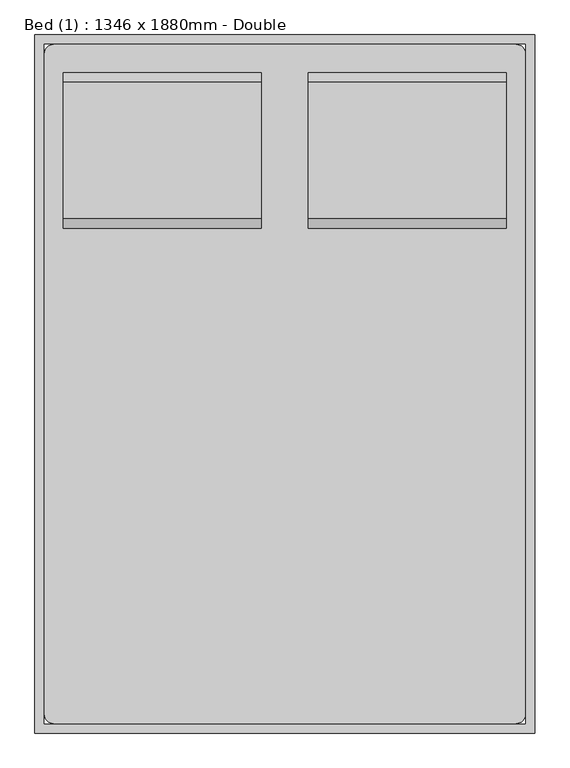
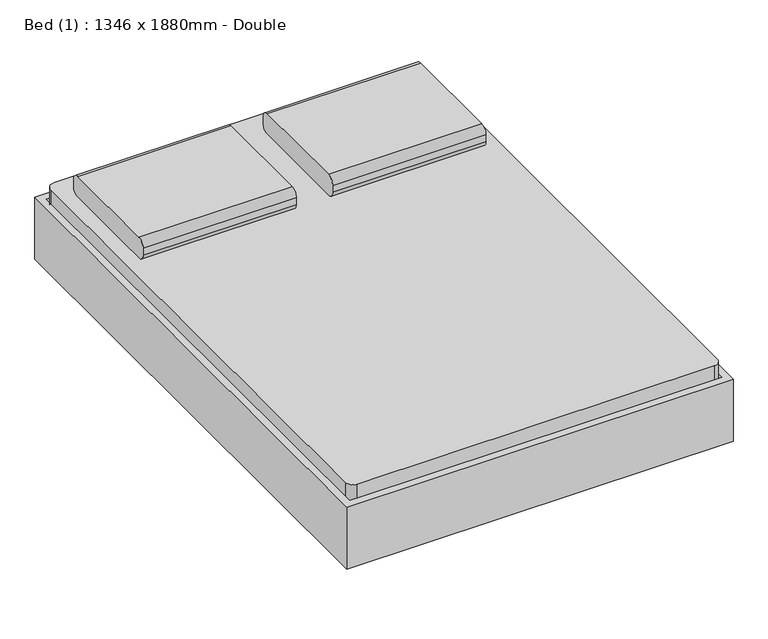
"""IFC4 building model written with IfcOpenShell, lengths in millimetres: furniture geometry, Bed (1) : 1346 x 1880mm - Double."""

from ifc_helpers import new_model, si_unit, point, frame, frame_2d, origin, place, context, project, spatial, polyline, circle_curve, trimmed, segment, composite_curve, outline, extrude, source, transform, mapped, element, save
from ifc_brep_helpers import plane_surface, cylinder_surface, revolved_surface, advanced_brep


def bed_1_1346_x_1880mm_double_99e58f25(model_context):
    return source(origin(), model_context, "Body", "SolidModel", [
        advanced_brep(
        [(-308.447541, -869.6295082, 196.85), (-308.447541, -869.6295082, 177.8), (-308.447541, -945.8295082, 177.8), (-308.447541, -945.8295082, 196.85), (-245.5113525, -869.6295082, 196.85), (-257.647541, -869.6295082, 177.8), (-257.647541, -945.8295082, 177.8), (-245.5113525, -945.8295082, 196.85), (-164.3115092, -869.6295082, 22.716374), (-181.5766725, -869.6295082, 14.6654962), (-181.5766725, -945.8295082, 14.6654962), (-164.3115092, -945.8295082, 22.716374), (-158.5564547, -869.6295082, 0.0), (-158.5564547, -869.6295082, 19.05), (-158.5564547, -945.8295082, 0.0), (-158.5564547, -945.8295082, 19.05), (-79.9439489, -869.6295082, 19.05), (-79.9439489, -869.6295082, 0.0), (-79.9439489, -945.8295082, 0.0), (-79.9439489, -945.8295082, 19.05), (-67.2439489, -869.6295082, 3.4029547), (-76.7689489, -869.6295082, 19.9007387), (-67.2439489, -945.8295082, 3.4029547), (-76.7689489, -945.8295082, 19.9007387), (-12.2513357, -869.6295082, 57.15), (-7.1469036, -869.6295082, 38.1), (-7.1469036, -945.8295082, 38.1), (-12.2513357, -945.8295082, 57.15), (690.5562537, -869.6295082, 57.15), (685.4518216, -869.6295082, 38.1), (685.4518216, -945.8295082, 38.1), (690.5562537, -945.8295082, 57.15), (755.0738669, -869.6295082, 19.9007387), (745.5488669, -869.6295082, 3.4029547), (745.5488669, -945.8295082, 3.4029547), (755.0738669, -945.8295082, 19.9007387), (758.2488669, -869.6295082, 0.0), (758.2488669, -869.6295082, 19.05), (758.2488669, -945.8295082, 0.0), (758.2488669, -945.8295082, 19.05), (836.8613728, -869.6295082, 19.05), (836.8613728, -869.6295082, 0.0), (836.8613728, -945.8295082, 0.0), (836.8613728, -945.8295082, 19.05), (859.8815906, -869.6295082, 14.6654962), (842.6164272, -869.6295082, 22.716374), (859.8815906, -945.8295082, 14.6654962), (842.6164272, -945.8295082, 22.716374), (923.8162705, -869.6295082, 196.85), (935.952459, -869.6295082, 177.8), (935.952459, -945.8295082, 177.8), (923.8162705, -945.8295082, 196.85), (986.752459, -869.6295082, 196.85), (986.752459, -945.8295082, 196.85), (986.752459, -945.8295082, 177.8), (986.752459, -869.6295082, 177.8)],
        [
            (0, 1),
            (1, 2),
            (2, 3),
            (3, 0),
            (0, 4),
            (4, 5),
            (5, 1),
            (5, 6),
            (6, 2),
            (6, 7),
            (7, 3),
            (7, 4),
            (4, 8),
            (8, 9),
            (9, 5),
            (9, 10),
            (10, 6),
            (10, 11),
            (11, 7),
            (11, 8),
            (12, 9, circle_curve(frame((-158.5564547, -869.6295082, 25.4), z_axis=(0.0, 1.0, 0.0), x_axis=(-0.906307787036664, 0.0, -0.4226182617406693)), 25.4)),
            (8, 13, circle_curve(frame((-158.5564547, -869.6295082, 25.4), z_axis=(0.0, -1.0, 0.0), x_axis=(-0.906307787036664, 0.0, -0.4226182617406693)), 6.35)),
            (13, 12),
            (14, 10, circle_curve(frame((-158.5564547, -945.8295082, 25.4), z_axis=(0.0, 1.0, 0.0), x_axis=(-0.906307787036664, 0.0, -0.4226182617406693)), 25.4)),
            (12, 14),
            (15, 11, circle_curve(frame((-158.5564547, -945.8295082, 25.4), z_axis=(0.0, 1.0, 0.0), x_axis=(-0.906307787036664, 0.0, -0.4226182617406693)), 6.35)),
            (14, 15),
            (15, 13),
            (13, 16),
            (16, 17),
            (17, 12),
            (17, 18),
            (18, 14),
            (18, 19),
            (19, 15),
            (19, 16),
            (20, 17, circle_curve(frame((-79.9439489, -869.6295082, 25.4), z_axis=(0.0, 1.0, 0.0), x_axis=(0.0, 0.0, -1.0)), 25.4)),
            (16, 21, circle_curve(frame((-79.9439489, -869.6295082, 25.4), z_axis=(0.0, -1.0, 0.0), x_axis=(0.0, 0.0, -1.0)), 6.35)),
            (21, 20),
            (22, 18, circle_curve(frame((-79.9439489, -945.8295082, 25.4), z_axis=(0.0, 1.0, 0.0), x_axis=(0.0, 0.0, -1.0)), 25.4)),
            (20, 22),
            (23, 19, circle_curve(frame((-79.9439489, -945.8295082, 25.4), z_axis=(0.0, 1.0, 0.0), x_axis=(0.0, 0.0, -1.0)), 6.35)),
            (22, 23),
            (23, 21),
            (21, 24),
            (24, 25),
            (25, 20),
            (25, 26),
            (26, 22),
            (26, 27),
            (27, 23),
            (27, 24),
            (24, 28),
            (28, 29),
            (29, 25),
            (29, 30),
            (30, 26),
            (30, 31),
            (31, 27),
            (31, 28),
            (28, 32),
            (32, 33),
            (33, 29),
            (33, 34),
            (34, 30),
            (34, 35),
            (35, 31),
            (35, 32),
            (36, 33, circle_curve(frame((758.2488669, -869.6295082, 25.4), z_axis=(0.0, 1.0, 0.0), x_axis=(-0.5000000000000533, 0.0, -0.866025403784408)), 25.4)),
            (32, 37, circle_curve(frame((758.2488669, -869.6295082, 25.4), z_axis=(0.0, -1.0, 0.0), x_axis=(-0.5000000000000533, 0.0, -0.866025403784408)), 6.35)),
            (37, 36),
            (38, 34, circle_curve(frame((758.2488669, -945.8295082, 25.4), z_axis=(0.0, 1.0, 0.0), x_axis=(-0.5000000000000533, 0.0, -0.866025403784408)), 25.4)),
            (36, 38),
            (39, 35, circle_curve(frame((758.2488669, -945.8295082, 25.4), z_axis=(0.0, 1.0, 0.0), x_axis=(-0.5000000000000533, 0.0, -0.866025403784408)), 6.35)),
            (38, 39),
            (39, 37),
            (37, 40),
            (40, 41),
            (41, 36),
            (41, 42),
            (42, 38),
            (42, 43),
            (43, 39),
            (43, 40),
            (44, 41, circle_curve(frame((836.8613728, -869.6295082, 25.4), z_axis=(0.0, 1.0, 0.0), x_axis=(0.0, 0.0, -1.0)), 25.4)),
            (40, 45, circle_curve(frame((836.8613728, -869.6295082, 25.4), z_axis=(0.0, -1.0, 0.0), x_axis=(0.0, 0.0, -1.0)), 6.35)),
            (45, 44),
            (46, 42, circle_curve(frame((836.8613728, -945.8295082, 25.4), z_axis=(0.0, 1.0, 0.0), x_axis=(0.0, 0.0, -1.0)), 25.4)),
            (44, 46),
            (47, 43, circle_curve(frame((836.8613728, -945.8295082, 25.4), z_axis=(0.0, 1.0, 0.0), x_axis=(0.0, 0.0, -1.0)), 6.35)),
            (46, 47),
            (47, 45),
            (45, 48),
            (48, 49),
            (49, 44),
            (49, 50),
            (50, 46),
            (50, 51),
            (51, 47),
            (51, 48),
            (52, 53),
            (53, 54),
            (54, 55),
            (55, 52),
            (48, 52),
            (55, 49),
            (54, 50),
            (53, 51),
        ],
        [
            plane_surface(frame((-308.447541, -1174.4295082, -127.5947323), z_axis=(-1.0, 0.0, 0.0), x_axis=(0.0, 1.0, 0.0))),
            plane_surface(frame((-308.447541, -869.6295082, 196.85), z_axis=(0.0, 1.0, 0.0), x_axis=(1.0, 0.0, 0.0))),
            plane_surface(frame((-308.447541, -869.6295082, 177.8), z_axis=(0.0, 0.0, -1.0), x_axis=(1.0, 0.0, 0.0))),
            plane_surface(frame((-308.447541, -945.8295082, 177.8), z_axis=(0.0, -1.0, 0.0), x_axis=(1.0, 0.0, 0.0))),
            plane_surface(frame((-308.447541, -945.8295082, 196.85), z_axis=(0.0, 0.0, 1.0), x_axis=(1.0, 0.0, 0.0))),
            plane_surface(frame((-245.5113525, -869.6295082, 196.85), z_axis=(0.0, 1.0000000000000002, 0.0), x_axis=(0.4226182617406713, 0.0, -0.9063077870366631))),
            plane_surface(frame((-257.647541, -869.6295082, 177.8), z_axis=(-0.9063077870366631, 0.0, -0.4226182617406712), x_axis=(0.4226182617406712, 0.0, -0.9063077870366631))),
            plane_surface(frame((-257.647541, -945.8295082, 177.8), z_axis=(0.0, -1.0000000000000002, 0.0), x_axis=(0.4226182617406716, 0.0, -0.906307787036663))),
            plane_surface(frame((-245.5113525, -945.8295082, 196.85), z_axis=(0.906307787036663, 0.0, 0.4226182617406715), x_axis=(0.4226182617406715, 0.0, -0.906307787036663))),
            plane_surface(frame((-158.5564547, -869.6295082, 25.4), z_axis=(0.0, 1.0, 0.0), x_axis=(-0.906307787036664, 0.0, -0.4226182617406693))),
            cylinder_surface(frame((-158.5564547, -1174.4295082, 25.4), z_axis=(0.0, -1.0, 0.0), x_axis=(-0.906307787036664, 0.0, -0.4226182617406693)), 25.4),
            plane_surface(frame((-158.5564547, -945.8295082, 25.4), z_axis=(0.0, -1.0, 0.0), x_axis=(-0.906307787036664, 0.0, -0.4226182617406693))),
            revolved_surface(polyline([(-164.3115091476828, -945.8295082, 22.71637403794675), (-164.3115091476828, -869.6295082, 22.71637403794675)]), (-158.5564547, -1174.4295082, 25.4), (0.0, -1.0, 0.0)),
            plane_surface(frame((-158.5564547, -869.6295082, 19.05), z_axis=(0.0, 1.0, 0.0), x_axis=(1.0, 0.0, 0.0))),
            plane_surface(frame((-158.5564547, -869.6295082, 0.0), z_axis=(0.0, 0.0, -1.0), x_axis=(1.0, 0.0, 0.0))),
            plane_surface(frame((-158.5564547, -945.8295082, 0.0), z_axis=(0.0, -1.0, 0.0), x_axis=(1.0, 0.0, 0.0))),
            plane_surface(frame((-158.5564547, -945.8295082, 19.05), z_axis=(0.0, 0.0, 1.0), x_axis=(1.0, 0.0, 0.0))),
            plane_surface(frame((-79.9439489, -869.6295082, 25.4), z_axis=(0.0, 1.0, 0.0), x_axis=(0.0, 0.0, -1.0))),
            cylinder_surface(frame((-79.9439489, -1174.4295082, 25.4), z_axis=(0.0, -1.0, 0.0), x_axis=(0.0, 0.0, -1.0)), 25.4),
            plane_surface(frame((-79.9439489, -945.8295082, 25.4), z_axis=(0.0, -1.0, 0.0), x_axis=(0.0, 0.0, -1.0))),
            revolved_surface(polyline([(-79.9439489, -945.8295082, 19.049999999999997), (-79.9439489, -869.6295082, 19.049999999999997)]), (-79.9439489, -1174.4295082, 25.4), (0.0, -1.0, 0.0)),
            plane_surface(frame((-76.7689489, -869.6295082, 19.9007387), z_axis=(0.0, 1.0, 0.0), x_axis=(0.8660254037844781, 0.0, 0.4999999999999317))),
            plane_surface(frame((-67.2439489, -869.6295082, 3.4029547), z_axis=(0.4999999999999313, 0.0, -0.8660254037844783), x_axis=(0.8660254037844783, 0.0, 0.4999999999999313))),
            plane_surface(frame((-67.2439489, -945.8295082, 3.4029547), z_axis=(0.0, -1.0000000000000002, 0.0), x_axis=(0.8660254037844788, 0.0, 0.49999999999993067))),
            plane_surface(frame((-76.7689489, -945.8295082, 19.9007387), z_axis=(-0.49999999999993067, 0.0, 0.8660254037844787), x_axis=(0.8660254037844787, 0.0, 0.49999999999993067))),
            plane_surface(frame((-12.2513357, -869.6295082, 57.15), z_axis=(0.0, 1.0, 0.0), x_axis=(1.0, 0.0, 0.0))),
            plane_surface(frame((-7.1469036, -869.6295082, 38.1), z_axis=(0.0, 0.0, -1.0), x_axis=(1.0, 0.0, 0.0))),
            plane_surface(frame((-7.1469036, -945.8295082, 38.1), z_axis=(0.0, -1.0, 0.0), x_axis=(1.0, 0.0, 0.0))),
            plane_surface(frame((-12.2513357, -945.8295082, 57.15), z_axis=(0.0, 0.0, 1.0), x_axis=(1.0, 0.0, 0.0))),
            plane_surface(frame((690.5562537, -869.6295082, 57.15), z_axis=(0.0, 1.0, 0.0), x_axis=(0.8660254037844102, 0.0, -0.5000000000000493))),
            plane_surface(frame((685.4518216, -869.6295082, 38.1), z_axis=(-0.500000000000049, 0.0, -0.8660254037844105), x_axis=(0.8660254037844105, 0.0, -0.500000000000049))),
            plane_surface(frame((685.4518216, -945.8295082, 38.1), z_axis=(0.0, -1.0, 0.0), x_axis=(0.8660254037844105, 0.0, -0.5000000000000488))),
            plane_surface(frame((690.5562537, -945.8295082, 57.15), z_axis=(0.5000000000000491, 0.0, 0.8660254037844103), x_axis=(0.8660254037844103, 0.0, -0.5000000000000491))),
            plane_surface(frame((758.2488669, -869.6295082, 25.4), z_axis=(0.0, 1.0, 0.0), x_axis=(-0.5000000000000533, 0.0, -0.866025403784408))),
            cylinder_surface(frame((758.2488669, -1174.4295082, 25.4), z_axis=(0.0, -1.0, 0.0), x_axis=(-0.5000000000000533, 0.0, -0.866025403784408)), 25.4),
            plane_surface(frame((758.2488669, -945.8295082, 25.4), z_axis=(0.0, -1.0, 0.0), x_axis=(-0.5000000000000533, 0.0, -0.866025403784408))),
            revolved_surface(polyline([(755.0738668999998, -945.8295082, 19.90073868596901), (755.0738668999998, -869.6295082, 19.90073868596901)]), (758.2488669, -1174.4295082, 25.4), (0.0, -1.0, 0.0)),
            plane_surface(frame((758.2488669, -869.6295082, 19.05), z_axis=(0.0, 1.0, 0.0), x_axis=(1.0, 0.0, 0.0))),
            plane_surface(frame((758.2488669, -869.6295082, 0.0), z_axis=(0.0, 0.0, -1.0), x_axis=(1.0, 0.0, 0.0))),
            plane_surface(frame((758.2488669, -945.8295082, 0.0), z_axis=(0.0, -1.0, 0.0), x_axis=(1.0, 0.0, 0.0))),
            plane_surface(frame((758.2488669, -945.8295082, 19.05), z_axis=(0.0, 0.0, 1.0), x_axis=(1.0, 0.0, 0.0))),
            plane_surface(frame((836.8613728, -869.6295082, 25.4), z_axis=(0.0, 1.0, 0.0), x_axis=(0.0, 0.0, -1.0))),
            cylinder_surface(frame((836.8613728, -1174.4295082, 25.4), z_axis=(0.0, -1.0, 0.0), x_axis=(0.0, 0.0, -1.0)), 25.4),
            plane_surface(frame((836.8613728, -945.8295082, 25.4), z_axis=(0.0, -1.0, 0.0), x_axis=(0.0, 0.0, -1.0))),
            revolved_surface(polyline([(836.8613728, -945.8295082, 19.049999999999997), (836.8613728, -869.6295082, 19.049999999999997)]), (836.8613728, -1174.4295082, 25.4), (0.0, -1.0, 0.0)),
            plane_surface(frame((842.6164272, -869.6295082, 22.716374), z_axis=(0.0, 1.0000000000000002, 0.0), x_axis=(0.42261826174054035, 0.0, 0.9063077870367242))),
            plane_surface(frame((859.8815906, -869.6295082, 14.6654962), z_axis=(0.9063077870367245, 0.0, -0.42261826174053974), x_axis=(0.42261826174053974, 0.0, 0.9063077870367245))),
            plane_surface(frame((859.8815906, -945.8295082, 14.6654962), z_axis=(0.0, -1.0, 0.0), x_axis=(0.42261826174053996, 0.0, 0.9063077870367243))),
            plane_surface(frame((842.6164272, -945.8295082, 22.716374), z_axis=(-0.9063077870367245, 0.0, 0.4226182617405396), x_axis=(0.4226182617405396, 0.0, 0.9063077870367245))),
            plane_surface(frame((986.752459, -1174.4295082, -127.5947323), z_axis=(1.0, 0.0, 0.0), x_axis=(0.0, 1.0, 0.0))),
            plane_surface(frame((923.8162705, -869.6295082, 196.85), z_axis=(0.0, 1.0, 0.0), x_axis=(1.0, 0.0, 0.0))),
            plane_surface(frame((935.952459, -869.6295082, 177.8), z_axis=(0.0, 0.0, -1.0), x_axis=(1.0, 0.0, 0.0))),
            plane_surface(frame((935.952459, -945.8295082, 177.8), z_axis=(0.0, -1.0, 0.0), x_axis=(1.0, 0.0, 0.0))),
            plane_surface(frame((923.8162705, -945.8295082, 196.85), z_axis=(0.0, 0.0, 1.0), x_axis=(1.0, 0.0, 0.0))),
        ],
        [
            (0, [[1, 2, 3, 4]]),
            (1, [[-1, 5, 6, 7]]),
            (2, [[-2, -7, 8, 9]]),
            (3, [[-3, -9, 10, 11]]),
            (4, [[-4, -11, 12, -5]]),
            (5, [[-6, 13, 14, 15]]),
            (6, [[-8, -15, 16, 17]]),
            (7, [[-10, -17, 18, 19]]),
            (8, [[-12, -19, 20, -13]]),
            (9, [[21, -14, 22, 23]]),
            (10, [[24, -16, -21, 25]]),
            (11, [[26, -18, -24, 27]]),
            (12, [[-22, -20, -26, 28]]),
            (13, [[-23, 29, 30, 31]]),
            (14, [[-25, -31, 32, 33]]),
            (15, [[-27, -33, 34, 35]]),
            (16, [[-28, -35, 36, -29]]),
            (17, [[37, -30, 38, 39]]),
            (18, [[40, -32, -37, 41]]),
            (19, [[42, -34, -40, 43]]),
            (20, [[-38, -36, -42, 44]]),
            (21, [[-39, 45, 46, 47]]),
            (22, [[-41, -47, 48, 49]]),
            (23, [[-43, -49, 50, 51]]),
            (24, [[-44, -51, 52, -45]]),
            (25, [[-46, 53, 54, 55]]),
            (26, [[-48, -55, 56, 57]]),
            (27, [[-50, -57, 58, 59]]),
            (28, [[-52, -59, 60, -53]]),
            (29, [[-54, 61, 62, 63]]),
            (30, [[-56, -63, 64, 65]]),
            (31, [[-58, -65, 66, 67]]),
            (32, [[-60, -67, 68, -61]]),
            (33, [[69, -62, 70, 71]]),
            (34, [[72, -64, -69, 73]]),
            (35, [[74, -66, -72, 75]]),
            (36, [[-70, -68, -74, 76]]),
            (37, [[-71, 77, 78, 79]]),
            (38, [[-73, -79, 80, 81]]),
            (39, [[-75, -81, 82, 83]]),
            (40, [[-76, -83, 84, -77]]),
            (41, [[85, -78, 86, 87]]),
            (42, [[88, -80, -85, 89]]),
            (43, [[90, -82, -88, 91]]),
            (44, [[-86, -84, -90, 92]]),
            (45, [[-87, 93, 94, 95]]),
            (46, [[-89, -95, 96, 97]]),
            (47, [[-91, -97, 98, 99]]),
            (48, [[-92, -99, 100, -93]]),
            (49, [[101, 102, 103, 104]]),
            (50, [[-94, 105, -104, 106]]),
            (51, [[-96, -106, -103, 107]]),
            (52, [[-98, -107, -102, 108]]),
            (53, [[-100, -108, -101, -105]]),
        ],
    ),
        extrude(outline(composite_curve([segment(polyline([(-283.047541, 680.1704918), (961.352459, 680.1704918)]), True, "CONTINUOUS"), segment(trimmed(circle_curve(frame_2d((961.352459, 654.7704918)), 25.4), [point((961.352459, 680.1704918))], [point((986.752459, 654.7704918))], False, "CARTESIAN"), True, "CONTINUOUS"), segment(polyline([(986.752459, 654.7704918), (986.752459, -1123.6295082)]), True, "CONTINUOUS"), segment(trimmed(circle_curve(frame_2d((961.352459, -1123.6295082)), 25.4), [point((986.752459, -1123.6295082))], [point((961.352459, -1149.0295082))], False, "CARTESIAN"), True, "CONTINUOUS"), segment(polyline([(961.352459, -1149.0295082), (-283.047541, -1149.0295082)]), True, "CONTINUOUS"), segment(trimmed(circle_curve(frame_2d((-283.047541, -1123.6295082)), 25.4), [point((-283.047541, -1149.0295082))], [point((-308.447541, -1123.6295082))], False, "CARTESIAN"), True, "CONTINUOUS"), segment(polyline([(-308.447541, -1123.6295082), (-308.447541, 654.7704918)]), True, "CONTINUOUS"), segment(trimmed(circle_curve(frame_2d((-283.047541, 654.7704918)), 25.4), [point((-308.447541, 654.7704918))], [point((-283.047541, 680.1704918))], False, "CARTESIAN"), True, "CONTINUOUS")], self_intersect=False)), frame((0.0, 0.0, 203.2), z_axis=(0.0, 0.0, 1.0), x_axis=(1.0, 0.0, 0.0)), (0.0, 0.0, 1.0), 203.2),
        advanced_brep(
        [(-308.1231784, 451.5704918, 177.8), (-308.1231784, 375.3704918, 177.8), (-308.1231784, 375.3704918, 196.85), (-308.1231784, 451.5704918, 196.85), (-257.3231784, 451.5704918, 177.8), (-257.3231784, 375.3704918, 177.8), (-245.1869899, 375.3704918, 196.85), (-245.1869899, 451.5704918, 196.85), (-181.2523099, 451.5704918, 14.6654962), (-181.2523099, 375.3704918, 14.6654962), (-163.9871466, 375.3704918, 22.716374), (-163.9871466, 451.5704918, 22.716374), (-158.2320921, 375.3704918, 0.0), (-158.2320921, 451.5704918, 0.0), (-158.2320921, 375.3704918, 19.05), (-158.2320921, 451.5704918, 19.05), (-79.6195862, 451.5704918, 0.0), (-79.6195862, 375.3704918, 0.0), (-79.6195862, 375.3704918, 19.05), (-79.6195862, 451.5704918, 19.05), (-66.9195862, 375.3704918, 3.4029547), (-66.9195862, 451.5704918, 3.4029547), (-76.4445862, 375.3704918, 19.9007387), (-76.4445862, 451.5704918, 19.9007387), (-6.822541, 451.5704918, 38.1), (-6.822541, 375.3704918, 38.1), (-11.9269731, 375.3704918, 57.15), (-11.9269731, 451.5704918, 57.15), (685.4518216, 451.5704918, 38.1), (685.4518216, 375.3704918, 38.1), (690.5562537, 375.3704918, 57.15), (690.5562537, 451.5704918, 57.15), (745.5488669, 451.5704918, 3.4029547), (745.5488669, 375.3704918, 3.4029547), (755.0738669, 375.3704918, 19.9007387), (755.0738669, 451.5704918, 19.9007387), (758.2488669, 375.3704918, 0.0), (758.2488669, 451.5704918, 0.0), (758.2488669, 375.3704918, 19.05), (758.2488669, 451.5704918, 19.05), (836.8613728, 451.5704918, 0.0), (836.8613728, 375.3704918, 0.0), (836.8613728, 375.3704918, 19.05), (836.8613728, 451.5704918, 19.05), (859.8815906, 375.3704918, 14.6654962), (859.8815906, 451.5704918, 14.6654962), (842.6164272, 375.3704918, 22.716374), (842.6164272, 451.5704918, 22.716374), (935.952459, 451.5704918, 177.8), (935.952459, 375.3704918, 177.8), (923.8162705, 375.3704918, 196.85), (923.8162705, 451.5704918, 196.85), (986.752459, 451.5704918, 177.8), (986.752459, 451.5704918, 196.85), (986.752459, 375.3704918, 196.85), (986.752459, 375.3704918, 177.8)],
        [
            (0, 1),
            (1, 2),
            (2, 3),
            (3, 0),
            (0, 4),
            (4, 5),
            (5, 1),
            (5, 6),
            (6, 2),
            (6, 7),
            (7, 3),
            (7, 4),
            (4, 8),
            (8, 9),
            (9, 5),
            (9, 10),
            (10, 6),
            (10, 11),
            (11, 7),
            (11, 8),
            (12, 9, circle_curve(frame((-158.2320921, 375.3704918, 25.4), z_axis=(0.0, 1.0, 0.0), x_axis=(-0.906307787036649, 0.0, -0.4226182617407015)), 25.4)),
            (8, 13, circle_curve(frame((-158.2320921, 451.5704918, 25.4), z_axis=(0.0, -1.0, 0.0), x_axis=(-0.906307787036649, 0.0, -0.4226182617407015)), 25.4)),
            (13, 12),
            (14, 10, circle_curve(frame((-158.2320921, 375.3704918, 25.4), z_axis=(0.0, 1.0, 0.0), x_axis=(-0.906307787036649, 0.0, -0.4226182617407015)), 6.35)),
            (12, 14),
            (15, 11, circle_curve(frame((-158.2320921, 451.5704918, 25.4), z_axis=(0.0, 1.0, 0.0), x_axis=(-0.906307787036649, 0.0, -0.4226182617407015)), 6.35)),
            (14, 15),
            (15, 13),
            (13, 16),
            (16, 17),
            (17, 12),
            (17, 18),
            (18, 14),
            (18, 19),
            (19, 15),
            (19, 16),
            (20, 17, circle_curve(frame((-79.6195862, 375.3704918, 25.4), z_axis=(0.0, 1.0, 0.0), x_axis=(0.0, 0.0, -1.0)), 25.4)),
            (16, 21, circle_curve(frame((-79.6195862, 451.5704918, 25.4), z_axis=(0.0, -1.0, 0.0), x_axis=(0.0, 0.0, -1.0)), 25.4)),
            (21, 20),
            (22, 18, circle_curve(frame((-79.6195862, 375.3704918, 25.4), z_axis=(0.0, 1.0, 0.0), x_axis=(0.0, 0.0, -1.0)), 6.35)),
            (20, 22),
            (23, 19, circle_curve(frame((-79.6195862, 451.5704918, 25.4), z_axis=(0.0, 1.0, 0.0), x_axis=(0.0, 0.0, -1.0)), 6.35)),
            (22, 23),
            (23, 21),
            (21, 24),
            (24, 25),
            (25, 20),
            (25, 26),
            (26, 22),
            (26, 27),
            (27, 23),
            (27, 24),
            (24, 28),
            (28, 29),
            (29, 25),
            (29, 30),
            (30, 26),
            (30, 31),
            (31, 27),
            (31, 28),
            (28, 32),
            (32, 33),
            (33, 29),
            (33, 34),
            (34, 30),
            (34, 35),
            (35, 31),
            (35, 32),
            (36, 33, circle_curve(frame((758.2488669, 375.3704918, 25.4), z_axis=(0.0, 1.0, 0.0), x_axis=(-0.5000000000000449, 0.0, -0.8660254037844127)), 25.4)),
            (32, 37, circle_curve(frame((758.2488669, 451.5704918, 25.4), z_axis=(0.0, -1.0, 0.0), x_axis=(-0.5000000000000449, 0.0, -0.8660254037844127)), 25.4)),
            (37, 36),
            (38, 34, circle_curve(frame((758.2488669, 375.3704918, 25.4), z_axis=(0.0, 1.0, 0.0), x_axis=(-0.5000000000000449, 0.0, -0.8660254037844127)), 6.35)),
            (36, 38),
            (39, 35, circle_curve(frame((758.2488669, 451.5704918, 25.4), z_axis=(0.0, 1.0, 0.0), x_axis=(-0.5000000000000449, 0.0, -0.8660254037844127)), 6.35)),
            (38, 39),
            (39, 37),
            (37, 40),
            (40, 41),
            (41, 36),
            (41, 42),
            (42, 38),
            (42, 43),
            (43, 39),
            (43, 40),
            (44, 41, circle_curve(frame((836.8613728, 375.3704918, 25.4), z_axis=(0.0, 1.0, 0.0), x_axis=(0.0, 0.0, -1.0)), 25.4)),
            (40, 45, circle_curve(frame((836.8613728, 451.5704918, 25.4), z_axis=(0.0, -1.0, 0.0), x_axis=(0.0, 0.0, -1.0)), 25.4)),
            (45, 44),
            (46, 42, circle_curve(frame((836.8613728, 375.3704918, 25.4), z_axis=(0.0, 1.0, 0.0), x_axis=(0.0, 0.0, -1.0)), 6.35)),
            (44, 46),
            (47, 43, circle_curve(frame((836.8613728, 451.5704918, 25.4), z_axis=(0.0, 1.0, 0.0), x_axis=(0.0, 0.0, -1.0)), 6.35)),
            (46, 47),
            (47, 45),
            (45, 48),
            (48, 49),
            (49, 44),
            (49, 50),
            (50, 46),
            (50, 51),
            (51, 47),
            (51, 48),
            (52, 53),
            (53, 54),
            (54, 55),
            (55, 52),
            (48, 52),
            (55, 49),
            (54, 50),
            (53, 51),
        ],
        [
            plane_surface(frame((-308.1231784, 705.5704918, -152.9490627), z_axis=(-1.0, 0.0, 0.0), x_axis=(0.0, 1.0, 0.0))),
            plane_surface(frame((-308.1231784, 451.5704918, 177.8), z_axis=(0.0, 0.0, -1.0), x_axis=(1.0, 0.0, 0.0))),
            plane_surface(frame((-308.1231784, 375.3704918, 177.8), z_axis=(0.0, -1.0, 0.0), x_axis=(1.0, 0.0, 0.0))),
            plane_surface(frame((-308.1231784, 375.3704918, 196.85), z_axis=(0.0, 0.0, 1.0), x_axis=(1.0, 0.0, 0.0))),
            plane_surface(frame((-308.1231784, 451.5704918, 196.85), z_axis=(0.0, 1.0, 0.0), x_axis=(1.0, 0.0, 0.0))),
            plane_surface(frame((-257.3231784, 451.5704918, 177.8), z_axis=(-0.9063077870366483, 0.0, -0.4226182617407031), x_axis=(0.4226182617407031, 0.0, -0.9063077870366483))),
            plane_surface(frame((-257.3231784, 375.3704918, 177.8), z_axis=(0.0, -1.0, 0.0), x_axis=(0.4226182617407027, 0.0, -0.9063077870366485))),
            plane_surface(frame((-245.1869899, 375.3704918, 196.85), z_axis=(0.9063077870366484, 0.0, 0.4226182617407029), x_axis=(0.4226182617407029, 0.0, -0.9063077870366484))),
            plane_surface(frame((-245.1869899, 451.5704918, 196.85), z_axis=(0.0, 1.0, 0.0), x_axis=(0.4226182617407027, 0.0, -0.9063077870366485))),
            cylinder_surface(frame((-158.2320921, 705.5704918, 25.4), z_axis=(0.0, -1.0, 0.0), x_axis=(-0.906307787036649, 0.0, -0.4226182617407015)), 25.4),
            plane_surface(frame((-158.2320921, 375.3704918, 25.4), z_axis=(0.0, -1.0, 0.0), x_axis=(-0.906307787036649, 0.0, -0.4226182617407015))),
            revolved_surface(polyline([(-163.9871465476827, 375.3704918, 22.716374037946544), (-163.9871465476827, 451.5704918, 22.716374037946544)]), (-158.2320921, 705.5704918, 25.4), (0.0, -1.0, 0.0)),
            plane_surface(frame((-158.2320921, 451.5704918, 25.4), z_axis=(0.0, 1.0, 0.0), x_axis=(-0.906307787036649, 0.0, -0.4226182617407015))),
            plane_surface(frame((-158.2320921, 451.5704918, 0.0), z_axis=(0.0, 0.0, -1.0), x_axis=(1.0, 0.0, 0.0))),
            plane_surface(frame((-158.2320921, 375.3704918, 0.0), z_axis=(0.0, -1.0, 0.0), x_axis=(1.0, 0.0, 0.0))),
            plane_surface(frame((-158.2320921, 375.3704918, 19.05), z_axis=(0.0, 0.0, 1.0), x_axis=(1.0, 0.0, 0.0))),
            plane_surface(frame((-158.2320921, 451.5704918, 19.05), z_axis=(0.0, 1.0, 0.0), x_axis=(1.0, 0.0, 0.0))),
            cylinder_surface(frame((-79.6195862, 705.5704918, 25.4), z_axis=(0.0, -1.0, 0.0), x_axis=(0.0, 0.0, -1.0)), 25.4),
            plane_surface(frame((-79.6195862, 375.3704918, 25.4), z_axis=(0.0, -1.0, 0.0), x_axis=(0.0, 0.0, -1.0))),
            revolved_surface(polyline([(-79.6195862, 375.3704918, 19.049999999999997), (-79.6195862, 451.5704918, 19.049999999999997)]), (-79.6195862, 705.5704918, 25.4), (0.0, -1.0, 0.0)),
            plane_surface(frame((-79.6195862, 451.5704918, 25.4), z_axis=(0.0, 1.0, 0.0), x_axis=(0.0, 0.0, -1.0))),
            plane_surface(frame((-66.9195862, 451.5704918, 3.4029547), z_axis=(0.499999999999877, 0.0, -0.8660254037845097), x_axis=(0.8660254037845097, 0.0, 0.499999999999877))),
            plane_surface(frame((-66.9195862, 375.3704918, 3.4029547), z_axis=(0.0, -1.0, 0.0), x_axis=(0.8660254037845101, 0.0, 0.49999999999987615))),
            plane_surface(frame((-76.4445862, 375.3704918, 19.9007387), z_axis=(-0.4999999999998764, 0.0, 0.8660254037845101), x_axis=(0.8660254037845101, 0.0, 0.4999999999998764))),
            plane_surface(frame((-76.4445862, 451.5704918, 19.9007387), z_axis=(0.0, 1.0, 0.0), x_axis=(0.86602540378451, 0.0, 0.49999999999987643))),
            plane_surface(frame((-6.822541, 451.5704918, 38.1), z_axis=(0.0, 0.0, -1.0), x_axis=(1.0, 0.0, 0.0))),
            plane_surface(frame((-6.822541, 375.3704918, 38.1), z_axis=(0.0, -1.0, 0.0), x_axis=(1.0, 0.0, 0.0))),
            plane_surface(frame((-11.9269731, 375.3704918, 57.15), z_axis=(0.0, 0.0, 1.0), x_axis=(1.0, 0.0, 0.0))),
            plane_surface(frame((-11.9269731, 451.5704918, 57.15), z_axis=(0.0, 1.0, 0.0), x_axis=(1.0, 0.0, 0.0))),
            plane_surface(frame((685.4518216, 451.5704918, 38.1), z_axis=(-0.5000000000000447, 0.0, -0.866025403784413), x_axis=(0.866025403784413, 0.0, -0.5000000000000447))),
            plane_surface(frame((685.4518216, 375.3704918, 38.1), z_axis=(0.0, -1.0, 0.0), x_axis=(0.8660254037844118, 0.0, -0.5000000000000464))),
            plane_surface(frame((690.5562537, 375.3704918, 57.15), z_axis=(0.5000000000000462, 0.0, 0.8660254037844121), x_axis=(0.8660254037844121, 0.0, -0.5000000000000462))),
            plane_surface(frame((690.5562537, 451.5704918, 57.15), z_axis=(0.0, 1.0, 0.0), x_axis=(0.8660254037844126, 0.0, -0.5000000000000452))),
            cylinder_surface(frame((758.2488669, 705.5704918, 25.4), z_axis=(0.0, -1.0, 0.0), x_axis=(-0.5000000000000449, 0.0, -0.8660254037844127)), 25.4),
            plane_surface(frame((758.2488669, 375.3704918, 25.4), z_axis=(0.0, -1.0, 0.0), x_axis=(-0.5000000000000449, 0.0, -0.8660254037844127))),
            revolved_surface(polyline([(755.0738668999998, 375.3704918, 19.900738685968978), (755.0738668999998, 451.5704918, 19.900738685968978)]), (758.2488669, 705.5704918, 25.4), (0.0, -1.0, 0.0)),
            plane_surface(frame((758.2488669, 451.5704918, 25.4), z_axis=(0.0, 1.0, 0.0), x_axis=(-0.5000000000000449, 0.0, -0.8660254037844127))),
            plane_surface(frame((758.2488669, 451.5704918, 0.0), z_axis=(0.0, 0.0, -1.0), x_axis=(1.0, 0.0, 0.0))),
            plane_surface(frame((758.2488669, 375.3704918, 0.0), z_axis=(0.0, -1.0, 0.0), x_axis=(1.0, 0.0, 0.0))),
            plane_surface(frame((758.2488669, 375.3704918, 19.05), z_axis=(0.0, 0.0, 1.0), x_axis=(1.0, 0.0, 0.0))),
            plane_surface(frame((758.2488669, 451.5704918, 19.05), z_axis=(0.0, 1.0, 0.0), x_axis=(1.0, 0.0, 0.0))),
            cylinder_surface(frame((836.8613728, 705.5704918, 25.4), z_axis=(0.0, -1.0, 0.0), x_axis=(0.0, 0.0, -1.0)), 25.4),
            plane_surface(frame((836.8613728, 375.3704918, 25.4), z_axis=(0.0, -1.0, 0.0), x_axis=(0.0, 0.0, -1.0))),
            revolved_surface(polyline([(836.8613728, 375.3704918, 19.049999999999997), (836.8613728, 451.5704918, 19.049999999999997)]), (836.8613728, 705.5704918, 25.4), (0.0, -1.0, 0.0)),
            plane_surface(frame((836.8613728, 451.5704918, 25.4), z_axis=(0.0, 1.0, 0.0), x_axis=(0.0, 0.0, -1.0))),
            plane_surface(frame((859.8815906, 451.5704918, 14.6654962), z_axis=(0.9063077870366809, 0.0, -0.42261826174063316), x_axis=(0.42261826174063316, 0.0, 0.9063077870366809))),
            plane_surface(frame((859.8815906, 375.3704918, 14.6654962), z_axis=(0.0, -1.0, 0.0), x_axis=(0.4226182617406339, 0.0, 0.9063077870366806))),
            plane_surface(frame((842.6164272, 375.3704918, 22.716374), z_axis=(-0.906307787036681, 0.0, 0.422618261740633), x_axis=(0.422618261740633, 0.0, 0.906307787036681))),
            plane_surface(frame((842.6164272, 451.5704918, 22.716374), z_axis=(0.0, 1.0, 0.0), x_axis=(0.4226182617406331, 0.0, 0.9063077870366809))),
            plane_surface(frame((986.752459, 705.5704918, -152.9490627), z_axis=(1.0, 0.0, 0.0), x_axis=(0.0, 1.0, 0.0))),
            plane_surface(frame((935.952459, 451.5704918, 177.8), z_axis=(0.0, 0.0, -1.0), x_axis=(1.0, 0.0, 0.0))),
            plane_surface(frame((935.952459, 375.3704918, 177.8), z_axis=(0.0, -1.0, 0.0), x_axis=(1.0, 0.0, 0.0))),
            plane_surface(frame((923.8162705, 375.3704918, 196.85), z_axis=(0.0, 0.0, 1.0), x_axis=(1.0, 0.0, 0.0))),
            plane_surface(frame((923.8162705, 451.5704918, 196.85), z_axis=(0.0, 1.0, 0.0), x_axis=(1.0, 0.0, 0.0))),
        ],
        [
            (0, [[1, 2, 3, 4]]),
            (1, [[-1, 5, 6, 7]]),
            (2, [[-2, -7, 8, 9]]),
            (3, [[-3, -9, 10, 11]]),
            (4, [[-4, -11, 12, -5]]),
            (5, [[-6, 13, 14, 15]]),
            (6, [[-8, -15, 16, 17]]),
            (7, [[-10, -17, 18, 19]]),
            (8, [[-12, -19, 20, -13]]),
            (9, [[21, -14, 22, 23]]),
            (10, [[24, -16, -21, 25]]),
            (11, [[26, -18, -24, 27]]),
            (12, [[-22, -20, -26, 28]]),
            (13, [[-23, 29, 30, 31]]),
            (14, [[-25, -31, 32, 33]]),
            (15, [[-27, -33, 34, 35]]),
            (16, [[-28, -35, 36, -29]]),
            (17, [[37, -30, 38, 39]]),
            (18, [[40, -32, -37, 41]]),
            (19, [[42, -34, -40, 43]]),
            (20, [[-38, -36, -42, 44]]),
            (21, [[-39, 45, 46, 47]]),
            (22, [[-41, -47, 48, 49]]),
            (23, [[-43, -49, 50, 51]]),
            (24, [[-44, -51, 52, -45]]),
            (25, [[-46, 53, 54, 55]]),
            (26, [[-48, -55, 56, 57]]),
            (27, [[-50, -57, 58, 59]]),
            (28, [[-52, -59, 60, -53]]),
            (29, [[-54, 61, 62, 63]]),
            (30, [[-56, -63, 64, 65]]),
            (31, [[-58, -65, 66, 67]]),
            (32, [[-60, -67, 68, -61]]),
            (33, [[69, -62, 70, 71]]),
            (34, [[72, -64, -69, 73]]),
            (35, [[74, -66, -72, 75]]),
            (36, [[-70, -68, -74, 76]]),
            (37, [[-71, 77, 78, 79]]),
            (38, [[-73, -79, 80, 81]]),
            (39, [[-75, -81, 82, 83]]),
            (40, [[-76, -83, 84, -77]]),
            (41, [[85, -78, 86, 87]]),
            (42, [[88, -80, -85, 89]]),
            (43, [[90, -82, -88, 91]]),
            (44, [[-86, -84, -90, 92]]),
            (45, [[-87, 93, 94, 95]]),
            (46, [[-89, -95, 96, 97]]),
            (47, [[-91, -97, 98, 99]]),
            (48, [[-92, -99, 100, -93]]),
            (49, [[101, 102, 103, 104]]),
            (50, [[-94, 105, -104, 106]]),
            (51, [[-96, -106, -103, 107]]),
            (52, [[-98, -107, -102, 108]]),
            (53, [[-100, -108, -101, -105]]),
        ],
    ),
        extrude(outline(composite_curve([segment(polyline([(578.5704918, 406.4), (210.2704918, 406.4)]), True, "CONTINUOUS"), segment(trimmed(circle_curve(frame_2d((210.2704918, 431.8)), 25.4), [point((210.2704918, 406.4))], [point((184.8704918, 431.8))], False, "CARTESIAN"), True, "CONTINUOUS"), segment(polyline([(184.8704918, 431.8), (184.8704918, 457.2)]), True, "CONTINUOUS"), segment(trimmed(circle_curve(frame_2d((210.2704918, 457.2)), 25.4), [point((184.8704918, 457.2))], [point((210.2704918, 482.6))], False, "CARTESIAN"), True, "CONTINUOUS"), segment(polyline([(210.2704918, 482.6), (578.5704918, 482.6)]), True, "CONTINUOUS"), segment(trimmed(circle_curve(frame_2d((578.5704918, 457.2)), 25.4), [point((578.5704918, 482.6))], [point((603.9704918, 457.2))], False, "CARTESIAN"), True, "CONTINUOUS"), segment(polyline([(603.9704918, 457.2), (603.9704918, 431.8)]), True, "CONTINUOUS"), segment(trimmed(circle_curve(frame_2d((578.5704918, 431.8)), 25.4), [point((603.9704918, 431.8))], [point((578.5704918, 406.4))], False, "CARTESIAN"), True, "CONTINUOUS")], self_intersect=False)), frame((-257.647541, 0.0, 0.0), z_axis=(1.0, 0.0, 0.0), x_axis=(0.0, 1.0, 0.0)), (0.0, 0.0, 1.0), 533.3),
        extrude(outline(composite_curve([segment(polyline([(578.5704918, 406.4), (210.2704918, 406.4)]), True, "CONTINUOUS"), segment(trimmed(circle_curve(frame_2d((210.2704918, 431.8)), 25.4), [point((210.2704918, 406.4))], [point((184.8704918, 431.8))], False, "CARTESIAN"), True, "CONTINUOUS"), segment(polyline([(184.8704918, 431.8), (184.8704918, 457.2)]), True, "CONTINUOUS"), segment(trimmed(circle_curve(frame_2d((210.2704918, 457.2)), 25.4), [point((184.8704918, 457.2))], [point((210.2704918, 482.6))], False, "CARTESIAN"), True, "CONTINUOUS"), segment(polyline([(210.2704918, 482.6), (578.5704918, 482.6)]), True, "CONTINUOUS"), segment(trimmed(circle_curve(frame_2d((578.5704918, 457.2)), 25.4), [point((578.5704918, 482.6))], [point((603.9704918, 457.2))], False, "CARTESIAN"), True, "CONTINUOUS"), segment(polyline([(603.9704918, 457.2), (603.9704918, 431.8)]), True, "CONTINUOUS"), segment(trimmed(circle_curve(frame_2d((578.5704918, 431.8)), 25.4), [point((603.9704918, 431.8))], [point((578.5704918, 406.4))], False, "CARTESIAN"), True, "CONTINUOUS")], self_intersect=False)), frame((402.652459, 0.0, 0.0), z_axis=(1.0, 0.0, 0.0), x_axis=(0.0, 1.0, 0.0)), (0.0, 0.0, 1.0), 533.3),
        extrude(outline(polyline([(1012.152459, 705.5704918), (1012.152459, -1174.4295082), (-333.847541, -1174.4295082), (-333.847541, 705.5704918), (1012.152459, 705.5704918)]), holes=[polyline([(986.752459, 680.1704918), (-308.447541, 680.1704918), (-308.447541, -1149.0295082), (986.752459, -1149.0295082), (986.752459, 680.1704918)])]), frame((0.0, 0.0, 127.0), z_axis=(0.0, 0.0, 1.0), x_axis=(1.0, 0.0, 0.0)), (0.0, 0.0, 1.0), 228.6),
    ])


if __name__ == "__main__":
    model = new_model("IFC4")
    model_context = context("Model", 3, world=origin())
    ifc_project = project(units=[si_unit("LENGTHUNIT", "METRE", prefix="MILLI")], contexts=[model_context])
    site = spatial("IfcSite", under=ifc_project)
    building = spatial("IfcBuilding", under=site)
    placement = place(None, origin())
    bed_1_1346_x_1880mm_double_shape = bed_1_1346_x_1880mm_double_99e58f25(model_context)
    element("IfcFurniture", 1, ObjectType="Bed (1) : 1346 x 1880mm - Double", at=placement, inside=building, context=model_context, shape_type="MappedRepresentation", body=[
        mapped(bed_1_1346_x_1880mm_double_shape, transform((0.0, 0.0, 0.0), x_axis=(1.0, 0.0, 0.0), y_axis=(0.0, 1.0, 0.0), z_axis=(0.0, 0.0, 1.0))),
    ])
    save(model, "model.ifc")

# Revit data of these elements
# Type "Bed (1) : 1346 x 1880mm - Double"
#   Keynote = "N"
#   Length = 6' - 2.01575"
#   Width = 4' - 4.99213"
#   Material Frame = Wood - Birch
#   Material Mattress = Textile - White
#   Default Elevation = 0
# Element 1 (IfcFurniture, "Bed (1) : 1346 x 1880mm - Double")
#   Materials on its faces: "Wood - Birch", "Textile - White"
# Materials
#   "Wood - Birch": colour RGB 224 178 126, transparency 0
#   "Textile - White": colour RGB 247 247 239, transparency 0
